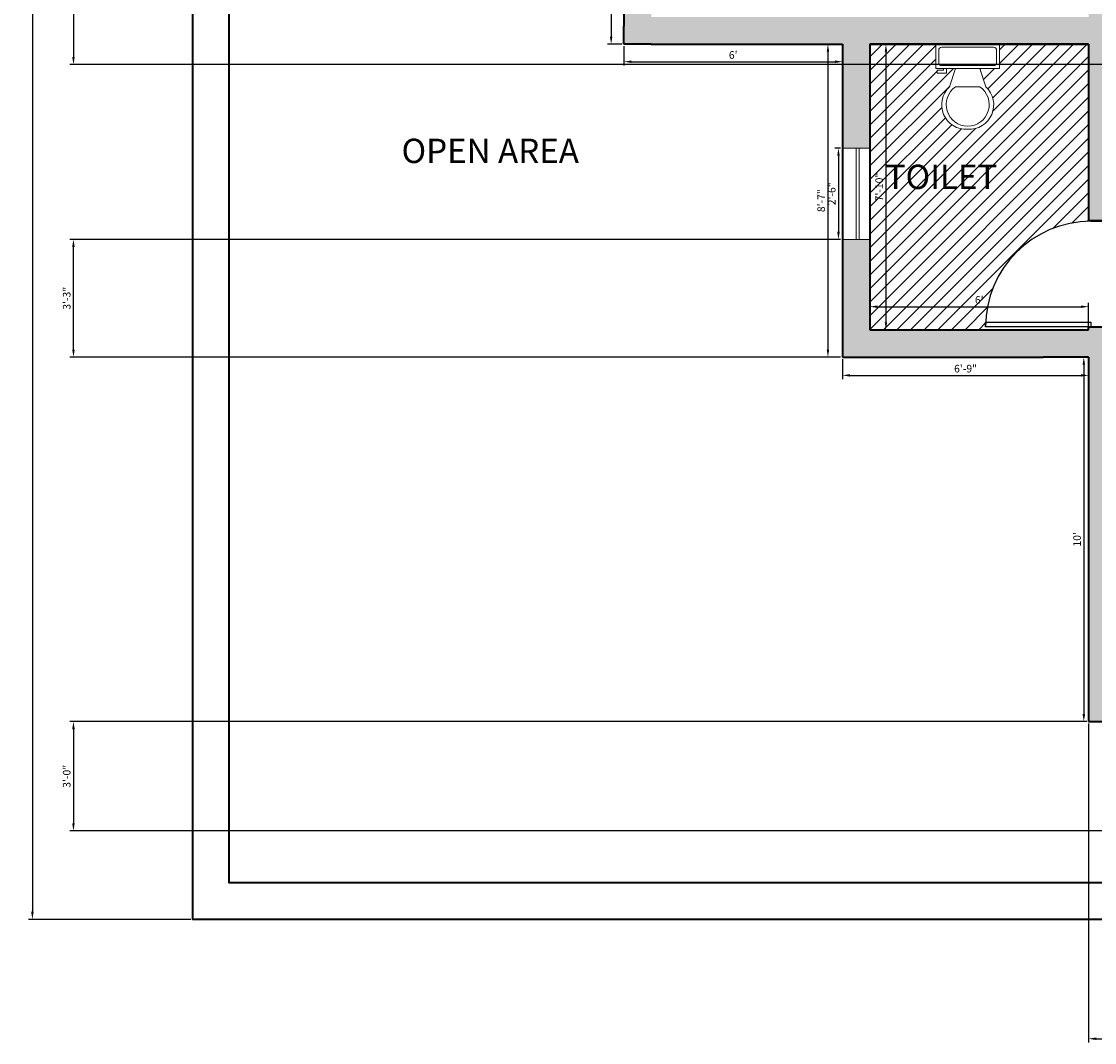
# Model space of a CAD drawing. Units: inches. Extents: x 2901 to 5923, y 918 to 2827.
# Tile 1 of 16: x 4232 to 4585, y 918 to 1254. Entities that reach past the tile are written whole.
import ezdxf

# ---------------------------------------------------------------- set-up
doc = ezdxf.new("R2010")
doc.units = ezdxf.units.IN
for name, color, linetype, lineweight in [('A-ANNO-DIMS', 2, 'Continuous', 18), ('A-AREA-IDEN', 7, 'Continuous', 25), ('A-FLOR-FIXT', 9, 'Continuous', 18), ('A-FLOR-PATT', 252, 'Continuous', 13), ('A-GLAZ', 4, 'Continuous', 18), ('A-WALL-PATT', 7, 'Continuous', 13), ('C-PROP', 7, 'Continuous', 35), ('doors', 240, 'Continuous', 25), ('walls', 7, 'Continuous', 35)]:
    doc.layers.add(name, color=color, linetype=linetype, lineweight=lineweight)
doc.styles.get("Standard").update_dxf_attribs({"font": 'arial.ttf'})
doc.dimstyles.new('Copy of ISO-25', dxfattribs={"dimtxt": 2.5, "dimasz": 2.5, "dimexe": 1.25, "dimexo": 0.625, "dimtad": 1, "dimdec": 1, "dimlunit": 4, "dimtxsty": 'Standard', "dimcen": 2.5, "dimadec": 0, "dimazin": 0, "dimtfac": 1, "dimtdec": 1, "dimtmove": 0, "dimatfit": 3, "dimfxl": 1, "dimarcsym": 0})

# ---------------------------------------------------------------- blocks, each defined once
blk = doc.blocks.new('*U6')
for p, q in [((0, 0), (0, -6)), ((40, 0), (40, -6))]:
    blk.add_line(p, q)
blk.add_lwpolyline([(0, 0), (0, 40), (1.75, 40), (1.75, 0)], close=True)
blk.add_arc((0, 0), 40, 0, 90)
blk = doc.blocks.new('*U20')
for p, q in [((241.3, -152.4), (241.3, -50.8)), ((-254, -215.9), (-203.2, -215.9)), ((-254, -241.3), (-254, -215.9)), ((-177.8, -241.3), (-254, -241.3)), ((-203.2, -215.9), (-203.2, -203.2)), ((-177.8, -203.2), (-177.8, -241.3)), ((-101.6, -203.2), (-152.4, -355.6)), ((101.6, -203.2), (152.4, -355.6)), ((101.6, -355.6), (-101.6, -355.6))]:
    blk.add_line(p, q)
blk.add_lwpolyline([(266.7, -203.2), (266.7, 0), (-266.7, 0), (-266.7, -203.2)], close=True)
for points in [[(-241.3, -50.8), (-241.3, -152.4)], [(215.9, -25.4), (-215.9, -25.4)], [(-215.9, -177.8), (215.9, -177.8)]]:
    blk.add_lwpolyline(points)
for centre, radius, start, end in [((-219.075, -47.625), 22.45064, 81.8699, 188.1301), ((219.075, -47.625), 22.45064, 351.8699, 98.1301), ((-219.075, -155.575), 22.45064, 171.869898, 278.1301), ((219.075, -155.575), 22.45064, 261.8699, 8.1301), ((-12.12088, -505.93752), 205.61935, 133.01722, 273.38), ((0.94996, -504.77674), 181.02486, 124.50543, 269.7), ((-0.94742, -504.77674), 181.02486, 270.3, 55.4946), ((12.12342, -505.93752), 205.61935, 266.62, 46.9828)]:
    blk.add_arc(centre, radius, start, end)
blk = doc.blocks.new('*D24')
at = {"layer": 'A-ANNO-DIMS', "color": 0, "lineweight": -2, "transparency": 16777216}
for p, q in [((4287.55, 1684.29), (4234.11, 1684.29)), ((4235.36, 1681.79), (4235.36, 960.79)), ((4287.55, 958.29), (4234.11, 958.29))]:
    blk.add_line(p, q, dxfattribs=at)
at = {"layer": 'A-ANNO-DIMS', "color": 0, "transparency": 16777216}
for points in [[(4234.95, 1681.79), (4235.78, 1681.79), (4235.36, 1684.29)], [(4234.95, 960.79), (4235.78, 960.79), (4235.36, 958.29)]]:
    blk.add_solid(points, dxfattribs=at)
at = {"layer": 'Defpoints', "color": 0, "transparency": 16777216}
for p in [(4288.18, 1684.29), (4235.36, 958.29), (4288.18, 958.29)]:
    blk.add_point(p, dxfattribs=at)
at = {"layer": 'A-ANNO-DIMS', "color": 0, "transparency": 16777216, "insert": (4233.46, 1321.29), "char_height": 2.5, "attachment_point": 5, "rotation": 90}
blk.add_mtext('60\'-6"', dxfattribs=at)
blk = doc.blocks.new('*D27')
at = {"layer": 'A-ANNO-DIMS', "color": 0, "lineweight": -2, "transparency": 16777216}
for p, q in [((4429.44, 1621.4), (4424.64, 1621.4)), ((4425.89, 1618.9), (4425.89, 1248.9)), ((4429.44, 1246.4), (4424.64, 1246.4))]:
    blk.add_line(p, q, dxfattribs=at)
at = {"layer": 'A-ANNO-DIMS', "color": 0, "transparency": 16777216}
for points in [[(4425.47, 1618.9), (4426.31, 1618.9), (4425.89, 1621.4)], [(4425.47, 1248.9), (4426.31, 1248.9), (4425.89, 1246.4)]]:
    blk.add_solid(points, dxfattribs=at)
at = {"layer": 'Defpoints', "color": 0, "transparency": 16777216}
for p in [(4430.07, 1621.4), (4425.89, 1246.4), (4430.07, 1246.4)]:
    blk.add_point(p, dxfattribs=at)
at = {"layer": 'A-ANNO-DIMS', "color": 0, "transparency": 16777216, "insert": (4423.99, 1433.9), "char_height": 2.5, "attachment_point": 5, "rotation": 90}
blk.add_mtext('31\'-3"', dxfattribs=at)
blk = doc.blocks.new('*D28')
at = {"layer": 'A-ANNO-DIMS', "color": 0, "lineweight": -2, "transparency": 16777216}
for p, q in [((4501.44, 1246.4), (4496.02, 1246.4)), ((4497.27, 1243.9), (4497.27, 1145.9)), ((4501.44, 1143.4), (4496.02, 1143.4))]:
    blk.add_line(p, q, dxfattribs=at)
at = {"layer": 'A-ANNO-DIMS', "color": 0, "transparency": 16777216}
for points in [[(4496.85, 1243.9), (4497.68, 1243.9), (4497.27, 1246.4)], [(4496.85, 1145.9), (4497.68, 1145.9), (4497.27, 1143.4)]]:
    blk.add_solid(points, dxfattribs=at)
at = {"layer": 'Defpoints', "color": 0, "transparency": 16777216}
for p in [(4502.07, 1246.4), (4497.27, 1143.4), (4502.07, 1143.4)]:
    blk.add_point(p, dxfattribs=at)
at = {"layer": 'A-ANNO-DIMS', "color": 0, "transparency": 16777216, "insert": (4495.37, 1194.9), "char_height": 2.5, "attachment_point": 5, "rotation": 90}
blk.add_mtext('8\'-7"', dxfattribs=at)
blk = doc.blocks.new('*D29')
at = {"layer": 'A-ANNO-DIMS', "color": 0, "lineweight": -2, "transparency": 16777216}
for p, q in [((4430.07, 1245.77), (4430.07, 1239.39)), ((4502.07, 1245.77), (4502.07, 1239.39)), ((4432.57, 1240.64), (4499.57, 1240.64))]:
    blk.add_line(p, q, dxfattribs=at)
at = {"layer": 'A-ANNO-DIMS', "color": 0, "transparency": 16777216}
for points in [[(4432.57, 1241.06), (4432.57, 1240.23), (4430.07, 1240.64)], [(4499.57, 1241.06), (4499.57, 1240.23), (4502.07, 1240.64)]]:
    blk.add_solid(points, dxfattribs=at)
at = {"layer": 'Defpoints', "color": 0, "transparency": 16777216}
for p in [(4430.07, 1246.4), (4502.07, 1246.4), (4502.07, 1240.64)]:
    blk.add_point(p, dxfattribs=at)
at = {"layer": 'A-ANNO-DIMS', "color": 0, "transparency": 16777216, "insert": (4466.07, 1242.54), "char_height": 2.5, "attachment_point": 5}
blk.add_mtext("6'", dxfattribs=at)
blk = doc.blocks.new('*D30')
at = {"layer": 'A-ANNO-DIMS', "color": 0, "lineweight": -2, "transparency": 16777216}
for p, q in [((4502.07, 1142.77), (4502.07, 1136.13)), ((4583.07, 1142.77), (4583.07, 1136.13)), ((4504.57, 1137.38), (4580.57, 1137.38))]:
    blk.add_line(p, q, dxfattribs=at)
at = {"layer": 'A-ANNO-DIMS', "color": 0, "transparency": 16777216}
for points in [[(4504.57, 1137.8), (4504.57, 1136.97), (4502.07, 1137.38)], [(4580.57, 1137.8), (4580.57, 1136.97), (4583.07, 1137.38)]]:
    blk.add_solid(points, dxfattribs=at)
at = {"layer": 'Defpoints', "color": 0, "transparency": 16777216}
for p in [(4502.07, 1143.4), (4583.07, 1143.4), (4583.07, 1137.38)]:
    blk.add_point(p, dxfattribs=at)
at = {"layer": 'A-ANNO-DIMS', "color": 0, "transparency": 16777216, "insert": (4542.57, 1139.28), "char_height": 2.5, "attachment_point": 5}
blk.add_mtext('6\'-9"', dxfattribs=at)
blk = doc.blocks.new('*D31')
at = {"layer": 'A-ANNO-DIMS', "color": 0, "lineweight": -2, "transparency": 16777216}
for p, q in [((4582.44, 1143.4), (4580.25, 1143.4)), ((4581.5, 1140.9), (4581.5, 1025.9)), ((4582.44, 1023.4), (4580.25, 1023.4))]:
    blk.add_line(p, q, dxfattribs=at)
at = {"layer": 'A-ANNO-DIMS', "color": 0, "transparency": 16777216}
for points in [[(4581.09, 1140.9), (4581.92, 1140.9), (4581.5, 1143.4)], [(4581.09, 1025.9), (4581.92, 1025.9), (4581.5, 1023.4)]]:
    blk.add_solid(points, dxfattribs=at)
at = {"layer": 'Defpoints', "color": 0, "transparency": 16777216}
for p in [(4583.07, 1143.4), (4581.5, 1023.4), (4583.07, 1023.4)]:
    blk.add_point(p, dxfattribs=at)
at = {"layer": 'A-ANNO-DIMS', "color": 0, "transparency": 16777216, "insert": (4579.6, 1083.4), "char_height": 2.5, "attachment_point": 5, "rotation": 90}
blk.add_mtext("10'", dxfattribs=at)
blk = doc.blocks.new('*D57')
at = {"layer": 'A-ANNO-DIMS', "color": 0, "lineweight": -2, "transparency": 16777216}
for p, q in [((4511.69, 1246.4), (4517.61, 1246.4)), ((4516.36, 1243.9), (4516.36, 1154.9)), ((4511.69, 1152.4), (4517.61, 1152.4))]:
    blk.add_line(p, q, dxfattribs=at)
at = {"layer": 'A-ANNO-DIMS', "color": 0, "transparency": 16777216}
for points in [[(4515.94, 1243.9), (4516.77, 1243.9), (4516.36, 1246.4)], [(4515.94, 1154.9), (4516.77, 1154.9), (4516.36, 1152.4)]]:
    blk.add_solid(points, dxfattribs=at)
at = {"layer": 'Defpoints', "color": 0, "transparency": 16777216}
for p in [(4511.07, 1246.4), (4511.07, 1152.4), (4516.36, 1152.4)]:
    blk.add_point(p, dxfattribs=at)
at = {"layer": 'A-ANNO-DIMS', "color": 0, "transparency": 16777216, "insert": (4514.45, 1199.4), "char_height": 2.5, "attachment_point": 5, "rotation": 90}
blk.add_mtext('7\'-10"', dxfattribs=at)
blk = doc.blocks.new('*D58')
at = {"layer": 'A-ANNO-DIMS', "color": 0, "lineweight": -2, "transparency": 16777216}
for p, q in [((4511.07, 1153.02), (4511.07, 1161.25)), ((4513.57, 1160), (4580.57, 1160)), ((4583.07, 1153.02), (4583.07, 1161.25))]:
    blk.add_line(p, q, dxfattribs=at)
at = {"layer": 'A-ANNO-DIMS', "color": 0, "transparency": 16777216}
for points in [[(4513.57, 1160.41), (4513.57, 1159.58), (4511.07, 1160)], [(4580.57, 1160.41), (4580.57, 1159.58), (4583.07, 1160)]]:
    blk.add_solid(points, dxfattribs=at)
at = {"layer": 'Defpoints', "color": 0, "transparency": 16777216}
for p in [(4583.07, 1160), (4511.07, 1152.4), (4583.07, 1152.4)]:
    blk.add_point(p, dxfattribs=at)
at = {"layer": 'A-ANNO-DIMS', "color": 0, "transparency": 16777216, "insert": (4547.07, 1161.9), "char_height": 2.5, "attachment_point": 5}
blk.add_mtext("6'", dxfattribs=at)
blk = doc.blocks.new('*D67')
at = {"layer": 'A-ANNO-DIMS', "color": 0, "lineweight": -2, "transparency": 16777216}
for p, q in [((4501.44, 1212.16), (4499.48, 1212.16)), ((4500.73, 1209.66), (4500.73, 1184.66)), ((4501.44, 1182.16), (4499.48, 1182.16))]:
    blk.add_line(p, q, dxfattribs=at)
at = {"layer": 'A-ANNO-DIMS', "color": 0, "transparency": 16777216}
for points in [[(4500.31, 1209.66), (4501.15, 1209.66), (4500.73, 1212.16)], [(4500.31, 1184.66), (4501.15, 1184.66), (4500.73, 1182.16)]]:
    blk.add_solid(points, dxfattribs=at)
at = {"layer": 'Defpoints', "color": 0, "transparency": 16777216}
for p in [(4502.07, 1212.16), (4500.73, 1182.16), (4502.07, 1182.16)]:
    blk.add_point(p, dxfattribs=at)
at = {"layer": 'A-ANNO-DIMS', "color": 0, "transparency": 16777216, "insert": (4498.83, 1197.16), "char_height": 2.5, "attachment_point": 5, "rotation": 90}
blk.add_mtext('2\'-6"', dxfattribs=at)
blk = doc.blocks.new('WIN-30')
for p, q in [((0, 30), (9, 30)), ((4.5, 30), (4.5, 0)), ((5.5, 30), (5.5, 0)), ((9, 30), (9, 0)), ((9, 0), (0, 0))]:
    blk.add_line(p, q)
blk = doc.blocks.new('*D98')
at = {"layer": 'A-ANNO-DIMS', "color": 0, "lineweight": -2, "transparency": 16777216}
for p, q in [((4501.44, 1182.16), (4247.63, 1182.16)), ((4248.88, 1145.9), (4248.88, 1179.66)), ((4501.44, 1143.4), (4247.63, 1143.4))]:
    blk.add_line(p, q, dxfattribs=at)
at = {"layer": 'A-ANNO-DIMS', "color": 0, "transparency": 16777216}
for points in [[(4248.46, 1179.66), (4249.3, 1179.66), (4248.88, 1182.16)], [(4248.46, 1145.9), (4249.3, 1145.9), (4248.88, 1143.4)]]:
    blk.add_solid(points, dxfattribs=at)
at = {"layer": 'Defpoints', "color": 0, "transparency": 16777216}
for p in [(4248.88, 1182.16), (4502.07, 1182.16), (4502.07, 1143.4)]:
    blk.add_point(p, dxfattribs=at)
at = {"layer": 'A-ANNO-DIMS', "color": 0, "transparency": 16777216, "insert": (4246.98, 1162.78), "char_height": 2.5, "attachment_point": 5, "rotation": 90}
blk.add_mtext('3\'-3"', dxfattribs=at)
blk = doc.blocks.new('*D103')
at = {"layer": 'A-ANNO-DIMS', "color": 0, "lineweight": -2, "transparency": 16777216}
for p, q in [((4583.07, 1022.77), (4583.07, 917.74)), ((4613.07, 986.77), (4613.07, 917.74)), ((4585.57, 918.99), (4610.57, 918.99))]:
    blk.add_line(p, q, dxfattribs=at)
at = {"layer": 'A-ANNO-DIMS', "color": 0, "transparency": 16777216}
for points in [[(4585.57, 919.41), (4585.57, 918.58), (4583.07, 918.99)], [(4610.57, 919.41), (4610.57, 918.58), (4613.07, 918.99)]]:
    blk.add_solid(points, dxfattribs=at)
at = {"layer": 'Defpoints', "color": 0, "transparency": 16777216}
for p in [(4583.07, 1023.4), (4613.07, 987.4), (4613.07, 918.99)]:
    blk.add_point(p, dxfattribs=at)
at = {"layer": 'A-ANNO-DIMS', "color": 0, "transparency": 16777216, "insert": (4598.07, 920.89), "char_height": 2.5, "attachment_point": 5}
blk.add_mtext('2\'-6"', dxfattribs=at)
blk = doc.blocks.new('*D104')
at = {"layer": 'A-ANNO-DIMS', "color": 0, "lineweight": -2, "transparency": 16777216}
for p, q in [((4582.44, 1023.4), (4247.63, 1023.4)), ((4248.88, 1020.9), (4248.88, 989.9)), ((4612.44, 987.4), (4247.63, 987.4))]:
    blk.add_line(p, q, dxfattribs=at)
at = {"layer": 'A-ANNO-DIMS', "color": 0, "transparency": 16777216}
for points in [[(4248.46, 1020.9), (4249.3, 1020.9), (4248.88, 1023.4)], [(4248.46, 989.9), (4249.3, 989.9), (4248.88, 987.4)]]:
    blk.add_solid(points, dxfattribs=at)
at = {"layer": 'Defpoints', "color": 0, "transparency": 16777216}
for p in [(4583.07, 1023.4), (4248.88, 987.4), (4613.07, 987.4)]:
    blk.add_point(p, dxfattribs=at)
at = {"layer": 'A-ANNO-DIMS', "color": 0, "transparency": 16777216, "insert": (4246.98, 1005.4), "char_height": 2.5, "attachment_point": 5, "rotation": 90}
blk.add_mtext('3\'-0"', dxfattribs=at)
blk = doc.blocks.new('*D106')
at = {"layer": 'A-ANNO-DIMS', "color": 0, "lineweight": -2, "transparency": 16777216}
for p, q in [((4588.44, 1297.4), (4247.63, 1297.4)), ((4248.88, 1294.9), (4248.88, 1242.24)), ((4651.2, 1239.74), (4247.63, 1239.74))]:
    blk.add_line(p, q, dxfattribs=at)
at = {"layer": 'A-ANNO-DIMS', "color": 0, "transparency": 16777216}
for points in [[(4248.46, 1294.9), (4249.3, 1294.9), (4248.88, 1297.4)], [(4248.46, 1242.24), (4249.3, 1242.24), (4248.88, 1239.74)]]:
    blk.add_solid(points, dxfattribs=at)
at = {"layer": 'Defpoints', "color": 0, "transparency": 16777216}
for p in [(4589.07, 1297.4), (4248.88, 1239.74), (4651.83, 1239.74)]:
    blk.add_point(p, dxfattribs=at)
at = {"layer": 'A-ANNO-DIMS', "color": 0, "transparency": 16777216, "insert": (4246.96, 1268.57), "char_height": 2.5, "attachment_point": 5, "rotation": 90}
blk.add_mtext('4\'-9 1/2"', dxfattribs=at)

msp = doc.modelspace()

# ---------------------------------------------------------------- hatches: boundary and pattern name
at = {"layer": 'A-FLOR-PATT'}
h = msp.add_hatch(dxfattribs=at)
h.set_pattern_fill('ANSI31', color=256)
h.paths.add_polyline_path([(4583.07, 1246.4), (4553.77, 1246.4), (4553.77, 1238.4), (4547.27, 1238.4), (4549.27, 1232.4, -0.702573), (4543.27, 1218.4, -0.70256), (4537.27, 1232.4), (4539.27, 1238.4), (4536.27, 1238.4), (4536.27, 1236.9), (4533.27, 1236.9), (4533.27, 1238.4), (4532.77, 1238.4), (4532.77, 1246.4), (4511.07, 1246.4), (4511.07, 1152.4), (4549.17, 1152.4, -0.415952), (4583.07, 1188.09)])
at = {"layer": 'A-WALL-PATT'}
h = msp.add_hatch(color=256, dxfattribs=at)
h.dxf.hatch_style = 1
h.paths.add_polyline_path([(4439.07, 1447.4), (4583.07, 1447.4), (4583.07, 1340.4), (4589.07, 1340.4), (4589.07, 1453.4), (4589.07, 1455.39), (4583.07, 1455.39), (4583.07, 1453.4), (4439.07, 1453.4), (4439.07, 1501.84), (4430.07, 1501.84), (4430.07, 1399.4), (4439.07, 1399.4)])
h.paths.add_polyline_path([(4439.07, 1621.4), (4487.07, 1621.4), (4487.07, 1630.4), (4430.07, 1630.4), (4430.07, 1561.84), (4439.07, 1561.84)])
h.paths.add_polyline_path([(4630.61, 1630.4), (4535.07, 1630.4), (4535.07, 1621.4), (4583.07, 1621.4), (4583.07, 1495.4), (4589.07, 1495.4), (4637.07, 1495.4), (4637.07, 1501.4), (4589.07, 1501.4), (4589.07, 1621.4), (4630.61, 1621.4)])
h.paths.add_polyline_path([(4892.07, 1630.4), (4690.61, 1630.4), (4690.61, 1621.4), (4733.07, 1621.4), (4733.07, 1564.4), (4739.07, 1564.4), (4739.07, 1621.4), (4883.07, 1621.4), (4883.07, 1528.4), (4739.07, 1528.4), (4733.07, 1528.4), (4733.07, 1501.4), (4685.07, 1501.4), (4685.07, 1495.4), (4739.07, 1495.4), (4739.07, 1519.4), (4787.07, 1519.4), (4787.07, 1423.4), (4739.07, 1423.4), (4739.07, 1456.67), (4733.07, 1456.67), (4733.07, 1340.4), (4739.07, 1340.4), (4739.07, 1417.4), (4787.07, 1417.4), (4793.07, 1417.4), (4793.07, 1423.4), (4793.07, 1519.4), (4883.07, 1519.4), (4883.07, 1482.87), (4892.07, 1482.87)])
h.paths.add_polyline_path([(4892.07, 1458.87), (4883.07, 1458.87), (4883.07, 1423.4), (4823.07, 1423.4), (4823.07, 1417.4), (4883.07, 1417.4), (4883.07, 1363.31), (4892.07, 1363.31)], flags=17)
h.paths.add_polyline_path([(4892.07, 1303.31), (4883.07, 1303.31), (4883.07, 1255.4), (4739.07, 1255.4), (4739.07, 1304.4), (4733.07, 1304.4), (4733.07, 1303.4), (4733.07, 1297.4), (4733.07, 1255.4), (4733.07, 1248.4), (4811.07, 1248.4), (4811.07, 1212.16), (4820.07, 1212.16), (4820.07, 1248.4), (4892.07, 1248.4)])
h.paths.add_polyline_path([(4820.07, 1182.16), (4811.07, 1182.16), (4811.07, 1152.4), (4685.07, 1152.4), (4685.07, 1147.03), (4685.07, 1143.4), (4733.07, 1143.4), (4811.07, 1143.4), (4814.07, 1143.4), (4820.07, 1143.4)])
h.paths.add_polyline_path([(4637.07, 1152.4), (4589.07, 1152.4), (4589.07, 1153.4), (4583.86, 1153.4), (4583.07, 1153.4), (4583.07, 1152.4), (4511.07, 1152.4), (4511.07, 1182.16), (4502.07, 1182.16), (4502.07, 1143.4), (4568.07, 1143.4), (4583.07, 1143.4), (4583.07, 1023.4), (4739.07, 1023.4), (4739.07, 1143.4), (4733.07, 1143.4), (4733.07, 1029.4), (4589.07, 1029.4), (4589.07, 1143.4), (4637.07, 1143.4), (4637.07, 1146.97)])
h.paths.add_polyline_path([(4511.07, 1246.4), (4583.07, 1246.4), (4583.07, 1188.4), (4589.07, 1188.4), (4589.07, 1246.4), (4589.07, 1248.4), (4589.07, 1255.4), (4589.07, 1297.4), (4697.07, 1297.4), (4697.07, 1303.4), (4589.07, 1303.4), (4589.07, 1304.4), (4583.07, 1304.4), (4583.07, 1255.4), (4439.07, 1255.4), (4439.07, 1261.4), (4439.07, 1351.4), (4430.07, 1351.4), (4430.07, 1252.4), (4430.07, 1246.4), (4439.07, 1246.4), (4487.07, 1246.4), (4502.07, 1246.4), (4502.07, 1212.16), (4511.07, 1212.16)])

# ---------------------------------------------------------------- linework, layer by layer
at = {"layer": 'C-PROP'}
msp.add_lwpolyline([(4288.18, 1684.29), (5015.18, 1684.29), (5015.18, 958.29), (4288.18, 958.29)], close=True, dxfattribs=at)
msp.add_lwpolyline([(5003.18, 978.26), (5003.18, 970.29), (4300.18, 970.29), (4300.18, 1672.29), (5003.18, 1672.29), (5003.18, 1132.27)], dxfattribs=at)
at = {"layer": 'walls'}
for p, q in [((4430.07, 1246.4), (4430.07, 1252.4)), ((4439.07, 1246.4), (4430.07, 1246.4)), ((4439.07, 1246.4), (4487.07, 1246.4)), ((4487.07, 1246.4), (4502.07, 1246.4)), ((4502.07, 1246.4), (4502.07, 1143.4)), ((4583.07, 1246.4), (4511.07, 1246.4)), ((4511.07, 1246.4), (4511.07, 1152.4)), ((4511.07, 1246.4), (4583.07, 1246.4)), ((4583.07, 1246.4), (4583.07, 1188.4)), ((4583.07, 1188.4), (4589.07, 1188.4)), ((4511.07, 1152.4), (4583.07, 1152.4)), ((4583.07, 1152.4), (4583.07, 1153.4)), ((4583.07, 1153.4), (4589.07, 1153.4)), ((4502.07, 1143.4), (4568.07, 1143.4)), ((4583.07, 1143.4), (4568.07, 1143.4)), ((4583.07, 1143.4), (4583.07, 1023.4)), ((4583.07, 1023.4), (4739.07, 1023.4))]:
    msp.add_line(p, q, dxfattribs=at)
msp.add_lwpolyline([(4892.07, 1630.4), (4430.07, 1630.4), (4430.07, 1252.4)], dxfattribs=at)

# ---------------------------------------------------------------- block references
at = {"layer": 'A-FLOR-FIXT', "xscale": 0.0393700787401575, "yscale": 0.0393700787401575, "zscale": 0.0393700787401575}
msp.add_blockref('*U20', (4543.27, 1246.4), dxfattribs=at)
at = {"layer": 'A-GLAZ'}
msp.add_blockref('WIN-30', (4502.07, 1182.16), dxfattribs=at)
at = {"layer": 'doors', "xscale": 0.8676351994906178, "yscale": 0.8676351994906178, "zscale": 0.8676351994906178, "rotation": 90}
msp.add_blockref('*U6', (4583.86, 1153.4), dxfattribs=at)

# ---------------------------------------------------------------- texts
at = {"layer": 'A-AREA-IDEN'}
for s, p in [('OPEN AREA', (4356.89, 1207.3)), ('TOILET', (4516.29, 1198.73))]:
    msp.add_text(s, height=8, dxfattribs=at).set_placement(p)

# ---------------------------------------------------------------- dimensions: what is measured, and where the dimension line sits
at = {"layer": 'A-ANNO-DIMS'}
for base, p1, p2, override, picture, middle in [((4235.36, 958.29), (4288.18, 1684.29), (4288.18, 958.29), {"dimclrd": 0, "dimclre": 0, "dimclrt": 0}, '*D24', (4233.46, 1321.29)), ((4425.89, 1246.4), (4430.07, 1621.4), (4430.07, 1246.4), {"dimclrd": 0, "dimclre": 0, "dimclrt": 0}, '*D27', (4423.99, 1433.9)), ((4248.88, 1239.74), (4589.07, 1297.4), (4651.83, 1239.74), {"dimdec": 1, "dimlfac": 1, "dimrnd": 0, "dimzin": 1, "dimdsep": 46, "dimlunit": 4, "dimfrac": 2}, '*D106', (4246.96, 1268.57)), ((4497.27, 1143.4), (4502.07, 1246.4), (4502.07, 1143.4), {"dimclrd": 0, "dimclre": 0, "dimclrt": 0}, '*D28', (4495.37, 1194.9)), ((4516.36, 1152.4), (4511.07, 1246.4), (4511.07, 1152.4), {"dimclrd": 0, "dimclre": 0, "dimclrt": 0}, '*D57', (4514.45, 1199.4)), ((4500.73, 1182.16), (4502.07, 1212.16), (4502.07, 1182.16), {"dimclrd": 0, "dimclre": 0, "dimclrt": 0}, '*D67', (4498.83, 1197.16)), ((4248.88, 1182.16), (4502.07, 1143.4), (4502.07, 1182.16), {"dimdec": 1, "dimlfac": 1, "dimrnd": 0, "dimzin": 1, "dimdsep": 46, "dimlunit": 4, "dimfrac": 2}, '*D98', (4246.98, 1162.78)), ((4581.5, 1023.4), (4583.07, 1143.4), (4583.07, 1023.4), {"dimclrd": 0, "dimclre": 0, "dimclrt": 0}, '*D31', (4579.6, 1083.4)), ((4248.88, 987.4), (4583.07, 1023.4), (4613.07, 987.4), {"dimdec": 1, "dimlfac": 1, "dimrnd": 0, "dimzin": 1, "dimdsep": 46, "dimlunit": 4, "dimfrac": 2}, '*D104', (4246.98, 1005.4))]:
    dim = msp.add_linear_dim(base=base, p1=p1, p2=p2, angle=90, dimstyle='Copy of ISO-25', override=override, dxfattribs=at)
    dim.commit()
    dim.dimension.update_dxf_attribs({"geometry": picture, "text_midpoint": middle})
for base, p1, p2, override, picture, middle in [((4502.07, 1240.64), (4430.07, 1246.4), (4502.07, 1246.4), {"dimclrd": 0, "dimclre": 0, "dimclrt": 0}, '*D29', (4466.07, 1242.54)), ((4583.07, 1160), (4511.07, 1152.4), (4583.07, 1152.4), {"dimclrd": 0, "dimclre": 0, "dimclrt": 0}, '*D58', (4547.07, 1161.9)), ((4583.07, 1137.38), (4502.07, 1143.4), (4583.07, 1143.4), {"dimclrd": 0, "dimclre": 0, "dimclrt": 0}, '*D30', (4542.57, 1139.28)), ((4613.07, 918.99), (4583.07, 1023.4), (4613.07, 987.4), {"dimdec": 1, "dimlfac": 1, "dimrnd": 0, "dimzin": 1, "dimdsep": 46, "dimlunit": 4, "dimfrac": 2}, '*D103', (4598.07, 920.89))]:
    dim = msp.add_linear_dim(base=base, p1=p1, p2=p2, dimstyle='Copy of ISO-25', override=override, dxfattribs=at)
    dim.commit()
    dim.dimension.update_dxf_attribs({"geometry": picture, "text_midpoint": middle})

doc.saveas('drawing.dxf')
